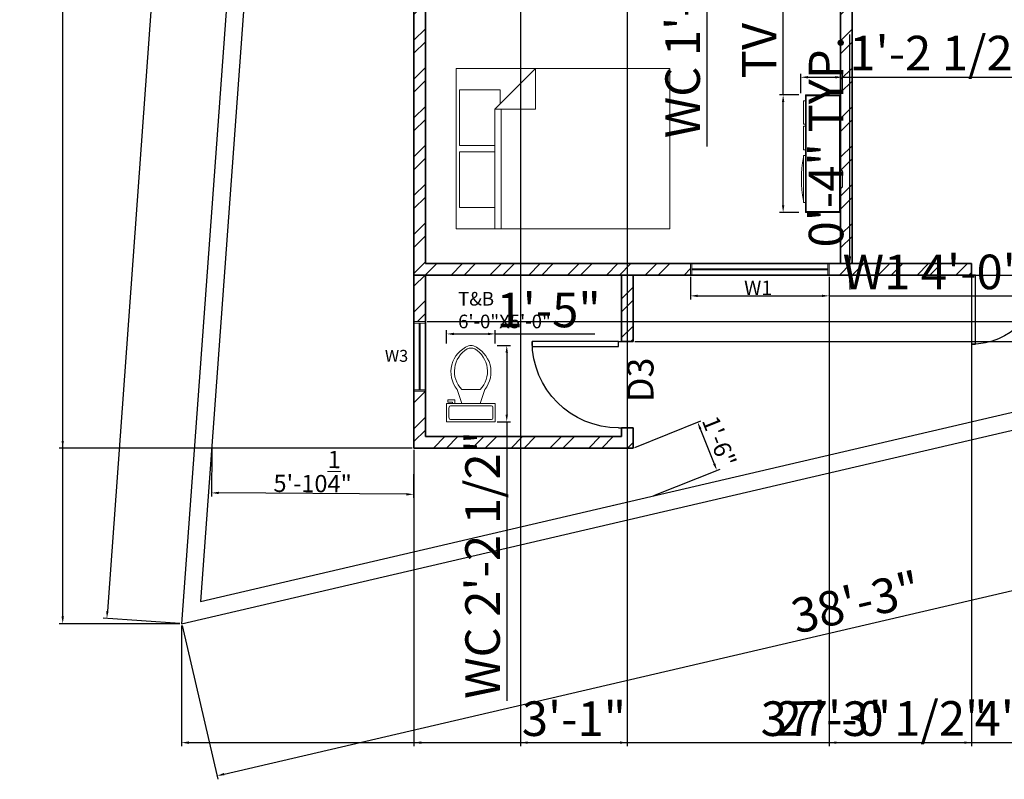
# Model space of a CAD drawing. Units: inches. Extents: x 2242 to 2870, y 1782 to 2635.
# Tile 1 of 7: x 2252 to 2594, y 1782 to 2046. Entities that reach past the tile are written whole.
import ezdxf

# ---------------------------------------------------------------- set-up
doc = ezdxf.new("R2010")
doc.units = ezdxf.units.IN
for name, color, linetype, lineweight in [('A-ANNO-DIMS', 7, 'Continuous', 18), ('A-ANNO-TEXT', 1, 'Continuous', 18), ('A-AREA-IDEN', 1, 'Continuous', 25), ('A-FLOR-FIXT', 9, 'Continuous', 18), ('A-WALL-PATT', 253, 'Continuous', 13), ('C-PROP', 7, 'Continuous', 30), ('doors', 5, 'Continuous', 25), ('furniture', 9, 'Continuous', 18), ('walls', 7, 'Continuous', 35), ('windows', 72, 'Continuous', 18)]:
    doc.layers.add(name, color=color, linetype=linetype, lineweight=lineweight)
doc.styles.get("Standard").update_dxf_attribs({"font": 'arial.ttf'})
doc.dimstyles.new('ISO-25', dxfattribs={"dimtxt": 12, "dimasz": 2.5, "dimexe": 1.25, "dimexo": 0.625, "dimtad": 1, "dimlunit": 4, "dimtxsty": 'Standard', "dimcen": 2.5, "dimadec": 0, "dimazin": 0, "dimtfac": 1, "dimtmove": 0, "dimatfit": 3, "dimfxl": 1, "dimarcsym": 0})

# ---------------------------------------------------------------- blocks, each defined once
blk = doc.blocks.new('*U2')
for p, q in [((0, 0), (0, -5)), ((30, 0), (30, -5))]:
    blk.add_line(p, q)
blk.add_lwpolyline([(0, 0), (0, 30), (1.75, 30), (1.75, 0)], close=True)
blk.add_arc((0, 0), 30, 0, 90)
blk = doc.blocks.new('Bed - Queen')
for p, q in [((0, -80.00003), (0, 0)), ((0, 0), (59.99999, 0)), ((59.99999, 0), (59.99999, -80.00003)), ((7.99999, -1.2), (28.79998, -1.2)), ((7.99999, -14.4), (7.99999, -1.2)), ((28.79998, -1.2), (28.79998, -14.4)), ((31.19999, -1.2), (51.99999, -1.2)), ((31.19999, -14.4), (31.19999, -1.2)), ((51.99999, -1.2), (51.99999, -16.4)), ((0, -14.4), (44.8, -14.4)), ((59.99999, -29.6), (44.8, -14.4)), ((44.8, -14.4), (44.8, -29.6)), ((44.8, -16.8), (0, -16.8)), ((51.99999, -16.4), (46.79936, -16.4)), ((44.8, -29.6), (59.99999, -29.6)), ((59.99999, -80.00003), (0, -80.00003))]:
    blk.add_line(p, q)
blk = doc.blocks.new('Toilet - top')
for p, q in [((9.5, -6), (9.5, -2)), ((-10, -8.5), (-8, -8.5)), ((-10, -9.5), (-10, -8.5)), ((-8, -8.5), (-8, -8)), ((-7, -8), (-7, -9.5)), ((-4, -8), (-6, -14)), ((4, -8), (6, -14)), ((-7, -9.5), (-10, -9.5)), ((4, -14), (-4, -14))]:
    blk.add_line(p, q)
blk.add_lwpolyline([(10.5, -8), (10.5, 0), (-10.5, 0), (-10.5, -8)], close=True)
for points in [[(-9.5, -2), (-9.5, -6)], [(8.5, -1), (-8.5, -1)], [(-8.5, -7), (8.5, -7)]]:
    blk.add_lwpolyline(points)
for centre, radius, start, end in [((-8.62, -1.88), 0.884, 81.8699, 188.1301), ((8.62, -1.88), 0.884, 351.8699, 98.1301), ((-8.62, -6.12), 0.884, 171.8699, 278.1301), ((8.62, -6.12), 0.884, 261.8699, 8.1301), ((3.52, -21.58), 12.17, 141.4691, 247.9714), ((4.2, -21.82), 11.33, 136.3677, 238.9468), ((-3.52, -21.58), 12.17, 292.0284, 38.5307), ((-4.2, -21.82), 11.33, 301.053, 43.6321), ((0, -27.88), 4, 245.7318, 294.2682), ((0, -29), 4, 254.8605, 285.1395)]:
    blk.add_arc(centre, radius, start, end)
blk = doc.blocks.new('Entertainment Center')
for p, q in [((-4, 0), (-5, -1)), ((4, 0), (-4, 0)), ((5, -1), (4, 0)), ((-17, -19), (-17, -1)), ((-17, -1), (43, -1)), ((-16.5, -18.5), (-16.5, -1.5)), ((-16.5, -1.5), (42.5, -1.5)), ((42.5, -1.5), (42.5, -18.5)), ((43, -1), (43, -19)), ((43, -19), (-17, -19)), ((42.5, -18.5), (-16.5, -18.5)), ((-12, -20), (-12, -19)), ((12, -20), (-12, -20)), ((12, -19), (12, -20)), ((15, -20), (15, -19)), ((27, -20), (15, -20)), ((27, -19), (27, -20)), ((28, -20), (28, -19)), ((40, -20), (28, -20)), ((40, -19), (40, -20))]:
    blk.add_line(p, q)
blk.add_arc((0, 40), 61, 259.6111, 280.3889)
blk = doc.blocks.new('*D16')
at = {"layer": 'A-ANNO-DIMS', "color": 0, "lineweight": -2, "transparency": 16777216}
for p, q in [((2358.54, 2540.38), (2331.98, 2542.3)), ((2333.04, 2539.72), (2282.38, 1840.55)), ((2307.51, 1836.23), (2280.95, 1838.15))]:
    blk.add_line(p, q, dxfattribs=at)
at = {"layer": 'A-ANNO-DIMS', "color": 0, "transparency": 16777216}
for points in [[(2332.63, 2539.75), (2333.46, 2539.69), (2333.22, 2542.21)], [(2281.96, 1840.58), (2282.79, 1840.52), (2282.2, 1838.06)]]:
    blk.add_solid(points, dxfattribs=at)
at = {"layer": 'Defpoints', "color": 0, "transparency": 16777216}
for p in [(2359.16, 2540.33), (2282.2, 1838.06), (2308.14, 1836.18)]:
    blk.add_point(p, dxfattribs=at)
at = {"layer": 'A-ANNO-DIMS', "color": 0, "transparency": 16777216, "insert": (2300.98, 2190.63), "char_height": 12, "attachment_point": 5, "rotation": 85.8553}
blk.add_mtext('58\'-10"', dxfattribs=at)
blk = doc.blocks.new('*D17')
at = {"layer": 'A-ANNO-DIMS', "color": 0, "lineweight": -2, "transparency": 16777216}
for p, q in [((2755.31, 1939.73), (2767.74, 1886.37)), ((2322.86, 1784), (2765.02, 1887.02)), ((2308.28, 1835.57), (2320.71, 1782.21))]:
    blk.add_line(p, q, dxfattribs=at)
at = {"layer": 'A-ANNO-DIMS', "color": 0, "transparency": 16777216}
for points in [[(2764.92, 1887.42), (2765.11, 1886.61), (2767.45, 1887.58)], [(2322.77, 1784.4), (2322.96, 1783.59), (2320.43, 1783.43)]]:
    blk.add_solid(points, dxfattribs=at)
at = {"layer": 'Defpoints', "color": 0, "transparency": 16777216}
for p in [(2755.16, 1940.33), (2767.45, 1887.58), (2308.14, 1836.18)]:
    blk.add_point(p, dxfattribs=at)
at = {"layer": 'A-ANNO-DIMS', "color": 0, "transparency": 16777216, "insert": (2542.41, 1842.09), "char_height": 12, "attachment_point": 5, "rotation": 13.1155}
blk.add_mtext('38\'-3"', dxfattribs=at)
blk = doc.blocks.new('*D18')
at = {"layer": 'A-ANNO-DIMS', "color": 0, "lineweight": -2, "transparency": 16777216}
for p, q in [((2465.32, 1897.33), (2488.32, 1906.52)), ((2488.08, 1903.73), (2492.91, 1891.67)), ((2472, 1880.62), (2495, 1889.81))]:
    blk.add_line(p, q, dxfattribs=at)
at = {"layer": 'A-ANNO-DIMS', "color": 0, "transparency": 16777216}
for points in [[(2488.47, 1903.89), (2487.7, 1903.58), (2487.16, 1906.06)], [(2493.29, 1891.82), (2492.52, 1891.51), (2493.84, 1889.34)]]:
    blk.add_solid(points, dxfattribs=at)
at = {"layer": 'Defpoints', "color": 0, "transparency": 16777216}
for p in [(2464.74, 1897.1), (2493.84, 1889.34), (2471.42, 1880.39)]:
    blk.add_point(p, dxfattribs=at)
at = {"layer": 'A-ANNO-DIMS', "color": 0, "transparency": 16777216, "insert": (2493.92, 1899.07), "char_height": 6, "attachment_point": 5, "rotation": 291.788}
blk.add_mtext('1\'-6"', dxfattribs=at)
blk = doc.blocks.new('*D20')
at = {"layer": 'A-ANNO-DIMS', "color": 0, "lineweight": -2, "transparency": 16777216}
for p, q in [((2318.6, 1896.99), (2318.48, 1880.3)), ((2388.74, 1896.47), (2388.62, 1879.78)), ((2386.13, 1881.05), (2320.99, 1881.53))]:
    blk.add_line(p, q, dxfattribs=at)
at = {"layer": 'A-ANNO-DIMS', "color": 0, "transparency": 16777216}
for points in [[(2320.99, 1881.95), (2320.98, 1881.11), (2318.49, 1881.55)], [(2386.13, 1881.47), (2386.12, 1880.63), (2388.63, 1881.03)]]:
    blk.add_solid(points, dxfattribs=at)
at = {"layer": 'Defpoints', "color": 0, "transparency": 16777216}
for p in [(2318.6, 1897.61), (2388.74, 1897.1), (2318.49, 1881.55)]:
    blk.add_point(p, dxfattribs=at)
at = {"layer": 'A-ANNO-DIMS', "color": 0, "transparency": 16777216, "insert": (2353.61, 1888.98), "char_height": 6, "attachment_point": 5, "rotation": 359.5783}
blk.add_mtext('5\'-10{\\H1x;\\S1/4;}"', dxfattribs=at)
blk = doc.blocks.new('WIN-W3-24IN')
for p, q in [((0, 0), (0, 24.12)), ((0, 24.12), (4, 24.12)), ((4, 24.12), (4, 0)), ((0, 23.62), (4, 23.62)), ((1.8, 23.62), (1.8, 0.5)), ((2.2, 23.62), (2.2, 0.5)), ((4, 0.5), (0, 0.5)), ((4, 0), (0, 0))]:
    blk.add_line(p, q)
blk = doc.blocks.new('WIN-W1-48IN')
for p, q in [((0, 4), (48.12, 4)), ((0, 0), (0, 4)), ((0.5, 0), (0.5, 4)), ((47.62, 4), (47.62, 0)), ((48.12, 4), (48.12, 0)), ((48.12, 0), (0, 0)), ((0.5, 2.2), (47.62, 2.2)), ((0.5, 1.8), (47.62, 1.8))]:
    blk.add_line(p, q)
blk = doc.blocks.new('*D35')
at = {"layer": 'A-ANNO-DIMS', "color": 0, "lineweight": -2, "transparency": 16777216}
for p, q in [((2484.67, 1956.47), (2484.67, 1948.63)), ((2532.79, 1956.47), (2532.79, 1948.63)), ((2487.17, 1949.88), (2530.29, 1949.88)), ((2532.79, 1949.88), (2639.98, 1949.88))]:
    blk.add_line(p, q, dxfattribs=at)
at = {"layer": 'A-ANNO-DIMS', "color": 0, "transparency": 16777216}
for points in [[(2487.17, 1950.3), (2487.17, 1949.46), (2484.67, 1949.88)], [(2530.29, 1950.3), (2530.29, 1949.46), (2532.79, 1949.88)]]:
    blk.add_solid(points, dxfattribs=at)
at = {"layer": 'Defpoints', "color": 0, "transparency": 16777216}
for p in [(2484.67, 1957.1), (2532.79, 1957.1), (2532.79, 1949.88)]:
    blk.add_point(p, dxfattribs=at)
at = {"layer": 'A-ANNO-DIMS', "color": 0, "transparency": 16777216, "insert": (2587.64, 1956.63), "char_height": 12, "attachment_point": 5}
blk.add_mtext('W1 4\'-0" TYP.', dxfattribs=at)
blk = doc.blocks.new('*D36')
at = {"layer": 'A-ANNO-DIMS', "color": 0, "lineweight": -2, "transparency": 16777216}
for p, q in [((2540.01, 1963.6), (2540.01, 2040.49)), ((2533.41, 1961.1), (2541.26, 1961.1)), ((2540.01, 1957.1), (2540.01, 1961.1)), ((2533.41, 1957.1), (2541.26, 1957.1)), ((2540.01, 1954.6), (2540.01, 1952.1))]:
    blk.add_line(p, q, dxfattribs=at)
at = {"layer": 'A-ANNO-DIMS', "color": 0, "transparency": 16777216}
for points in [[(2539.59, 1963.6), (2540.42, 1963.6), (2540.01, 1961.1)], [(2539.59, 1954.6), (2540.42, 1954.6), (2540.01, 1957.1)]]:
    blk.add_solid(points, dxfattribs=at)
at = {"layer": 'Defpoints', "color": 0, "transparency": 16777216}
for p in [(2532.79, 1961.1), (2540.01, 1961.1), (2532.79, 1957.1)]:
    blk.add_point(p, dxfattribs=at)
at = {"layer": 'A-ANNO-DIMS', "color": 0, "transparency": 16777216, "insert": (2533.26, 2003.3), "char_height": 12, "attachment_point": 5, "rotation": 90}
blk.add_mtext('0\'-4" TYP.', dxfattribs=at)
blk = doc.blocks.new('*D41')
at = {"layer": 'A-ANNO-DIMS', "color": 0, "lineweight": -2, "transparency": 16777216}
for p, q in [((2516.82, 2019.58), (2516.82, 2166.63)), ((2522.31, 2019.58), (2515.57, 2019.58)), ((2516.82, 1981.32), (2516.82, 2017.08)), ((2522.31, 1978.82), (2515.57, 1978.82))]:
    blk.add_line(p, q, dxfattribs=at)
at = {"layer": 'A-ANNO-DIMS', "color": 0, "transparency": 16777216}
for points in [[(2516.4, 2017.08), (2517.23, 2017.08), (2516.82, 2019.58)], [(2516.4, 1981.32), (2517.23, 1981.32), (2516.82, 1978.82)]]:
    blk.add_solid(points, dxfattribs=at)
at = {"layer": 'Defpoints', "color": 0, "transparency": 16777216}
for p in [(2516.82, 2019.58), (2522.93, 2019.58), (2522.93, 1978.82)]:
    blk.add_point(p, dxfattribs=at)
at = {"layer": 'A-ANNO-DIMS', "color": 0, "transparency": 16777216, "insert": (2510.06, 2094.35), "char_height": 12, "attachment_point": 5, "rotation": 90}
blk.add_mtext('TV UNIT 3\'-5" TYP.', dxfattribs=at)
blk = doc.blocks.new('*D42')
at = {"layer": 'A-ANNO-DIMS', "color": 0, "lineweight": -2, "transparency": 16777216}
for p, q in [((2522.93, 2020.21), (2522.93, 2026.94)), ((2525.43, 2025.69), (2534.92, 2025.69)), ((2537.42, 2020.21), (2537.42, 2026.94)), ((2537.42, 2025.69), (2641.15, 2025.69))]:
    blk.add_line(p, q, dxfattribs=at)
at = {"layer": 'A-ANNO-DIMS', "color": 0, "transparency": 16777216}
for points in [[(2525.43, 2026.11), (2525.43, 2025.28), (2522.93, 2025.69)], [(2534.92, 2026.11), (2534.92, 2025.28), (2537.42, 2025.69)]]:
    blk.add_solid(points, dxfattribs=at)
at = {"layer": 'Defpoints', "color": 0, "transparency": 16777216}
for p in [(2537.42, 2025.69), (2522.93, 2019.58), (2537.42, 2019.58)]:
    blk.add_point(p, dxfattribs=at)
at = {"layer": 'A-ANNO-DIMS', "color": 0, "transparency": 16777216, "insert": (2590.54, 2032.52), "char_height": 12, "attachment_point": 5}
blk.add_mtext('1\'-2 1/2" TYP.', dxfattribs=at)
blk = doc.blocks.new('*D47')
at = {"layer": 'A-ANNO-DIMS', "color": 0, "lineweight": -2, "transparency": 16777216}
for p, q in [((2417.57, 1932.69), (2422.18, 1932.69)), ((2420.93, 1930.19), (2420.93, 1908.65)), ((2417.57, 1906.15), (2422.18, 1906.15)), ((2420.93, 1906.15), (2420.93, 1809.46))]:
    blk.add_line(p, q, dxfattribs=at)
at = {"layer": 'A-ANNO-DIMS', "color": 0, "transparency": 16777216}
for points in [[(2420.51, 1930.19), (2421.35, 1930.19), (2420.93, 1932.69)], [(2420.51, 1908.65), (2421.35, 1908.65), (2420.93, 1906.15)]]:
    blk.add_solid(points, dxfattribs=at)
at = {"layer": 'Defpoints', "color": 0, "transparency": 16777216}
for p in [(2416.95, 1932.69), (2416.95, 1906.15), (2420.93, 1906.15)]:
    blk.add_point(p, dxfattribs=at)
at = {"layer": 'A-ANNO-DIMS', "color": 0, "transparency": 16777216, "insert": (2414.1, 1856.56), "char_height": 12, "attachment_point": 5, "rotation": 90}
blk.add_mtext('WC 2\'-2 1/2"', dxfattribs=at)
blk = doc.blocks.new('*D48')
at = {"layer": 'A-ANNO-DIMS', "color": 0, "lineweight": -2, "transparency": 16777216}
for p, q in [((2400.08, 1933.32), (2400.08, 1937.93)), ((2416.95, 1933.32), (2416.95, 1937.93)), ((2402.58, 1936.68), (2414.45, 1936.68)), ((2416.95, 1936.68), (2451.47, 1936.68))]:
    blk.add_line(p, q, dxfattribs=at)
at = {"layer": 'A-ANNO-DIMS', "color": 0, "transparency": 16777216}
for points in [[(2402.58, 1937.09), (2402.58, 1936.26), (2400.08, 1936.68)], [(2414.45, 1937.09), (2414.45, 1936.26), (2416.95, 1936.68)]]:
    blk.add_solid(points, dxfattribs=at)
at = {"layer": 'Defpoints', "color": 0, "transparency": 16777216}
for p in [(2416.95, 1936.68), (2400.08, 1932.69), (2416.95, 1932.69)]:
    blk.add_point(p, dxfattribs=at)
at = {"layer": 'A-ANNO-DIMS', "color": 0, "transparency": 16777216, "insert": (2435.46, 1943.43), "char_height": 12, "attachment_point": 5}
blk.add_mtext('1\'-5"', dxfattribs=at)
blk = doc.blocks.new('*D49')
at = {"layer": 'A-ANNO-DIMS', "color": 0, "lineweight": -2, "transparency": 16777216}
for p, q in [((2487.98, 2131.46), (2491.58, 2131.46)), ((2490.33, 2128.96), (2490.33, 2114.14)), ((2487.98, 2111.64), (2491.58, 2111.64)), ((2490.33, 2111.64), (2490.33, 2001.67))]:
    blk.add_line(p, q, dxfattribs=at)
at = {"layer": 'A-ANNO-DIMS', "color": 0, "transparency": 16777216}
for points in [[(2489.91, 2128.96), (2490.75, 2128.96), (2490.33, 2131.46)], [(2489.91, 2114.14), (2490.75, 2114.14), (2490.33, 2111.64)]]:
    blk.add_solid(points, dxfattribs=at)
at = {"layer": 'Defpoints', "color": 0, "transparency": 16777216}
for p in [(2487.36, 2131.46), (2487.36, 2111.64), (2490.33, 2111.64)]:
    blk.add_point(p, dxfattribs=at)
at = {"layer": 'A-ANNO-DIMS', "color": 0, "transparency": 16777216, "insert": (2483.5, 2055.41), "char_height": 12, "attachment_point": 5, "rotation": 90}
blk.add_mtext('WC 1\'-8" TYP.', dxfattribs=at)
blk = doc.blocks.new('*D55')
at = {"layer": 'A-ANNO-DIMS', "color": 0, "lineweight": -2, "transparency": 16777216}
for p, q in [((2358.54, 2540.33), (2265.64, 2540.33)), ((2266.89, 1838.68), (2266.89, 2537.83)), ((2307.51, 1836.18), (2265.64, 1836.18))]:
    blk.add_line(p, q, dxfattribs=at)
at = {"layer": 'A-ANNO-DIMS', "color": 0, "transparency": 16777216}
for points in [[(2266.47, 2537.83), (2267.3, 2537.83), (2266.89, 2540.33)], [(2266.47, 1838.68), (2267.3, 1838.68), (2266.89, 1836.18)]]:
    blk.add_solid(points, dxfattribs=at)
at = {"layer": 'Defpoints', "color": 0, "transparency": 16777216}
for p in [(2266.89, 2540.33), (2359.16, 2540.33), (2308.14, 1836.18)]:
    blk.add_point(p, dxfattribs=at)
at = {"layer": 'A-ANNO-DIMS', "color": 0, "transparency": 16777216, "insert": (2260.13, 2188.26), "char_height": 12, "attachment_point": 5, "rotation": 90}
blk.add_mtext('58\'-8"', dxfattribs=at)
blk = doc.blocks.new('*D56')
at = {"layer": 'A-ANNO-DIMS', "color": 0, "lineweight": -2, "transparency": 16777216}
for p, q in [((2755.16, 1939.71), (2755.16, 1793.68)), ((2308.14, 1835.56), (2308.14, 1793.68)), ((2310.64, 1794.93), (2752.66, 1794.93))]:
    blk.add_line(p, q, dxfattribs=at)
at = {"layer": 'A-ANNO-DIMS', "color": 0, "transparency": 16777216}
for points in [[(2310.64, 1795.35), (2310.64, 1794.51), (2308.14, 1794.93)], [(2752.66, 1795.35), (2752.66, 1794.51), (2755.16, 1794.93)]]:
    blk.add_solid(points, dxfattribs=at)
at = {"layer": 'Defpoints', "color": 0, "transparency": 16777216}
for p in [(2755.16, 1940.33), (2308.14, 1836.18), (2755.16, 1794.93)]:
    blk.add_point(p, dxfattribs=at)
at = {"layer": 'A-ANNO-DIMS', "color": 0, "transparency": 16777216, "insert": (2531.65, 1801.69), "char_height": 12, "attachment_point": 5}
blk.add_mtext('37\'-3"', dxfattribs=at)
blk = doc.blocks.new('*D57')
at = {"layer": 'A-ANNO-DIMS', "color": 0, "lineweight": -2, "transparency": 16777216}
for p, q in [((2713.16, 1956.47), (2713.16, 1793.68)), ((2388.74, 1896.47), (2388.74, 1793.68)), ((2391.24, 1794.93), (2710.66, 1794.93))]:
    blk.add_line(p, q, dxfattribs=at)
at = {"layer": 'A-ANNO-DIMS', "color": 0, "transparency": 16777216}
for points in [[(2391.24, 1795.35), (2391.24, 1794.51), (2388.74, 1794.93)], [(2710.66, 1795.35), (2710.66, 1794.51), (2713.16, 1794.93)]]:
    blk.add_solid(points, dxfattribs=at)
at = {"layer": 'Defpoints', "color": 0, "transparency": 16777216}
for p in [(2713.16, 1957.1), (2388.74, 1897.1), (2713.16, 1794.93)]:
    blk.add_point(p, dxfattribs=at)
at = {"layer": 'A-ANNO-DIMS', "color": 0, "transparency": 16777216, "insert": (2550.95, 1801.76), "char_height": 12, "attachment_point": 5}
blk.add_mtext('27\'-0 1/2"', dxfattribs=at)
blk = doc.blocks.new('*D58')
at = {"layer": 'A-ANNO-DIMS', "color": 0, "lineweight": -2, "transparency": 16777216}
for p, q in [((2388.12, 2433.1), (2265.64, 2433.1)), ((2266.89, 1899.6), (2266.89, 2430.6)), ((2388.12, 1897.1), (2265.64, 1897.1))]:
    blk.add_line(p, q, dxfattribs=at)
at = {"layer": 'A-ANNO-DIMS', "color": 0, "transparency": 16777216}
for points in [[(2266.47, 2430.6), (2267.3, 2430.6), (2266.89, 2433.1)], [(2266.47, 1899.6), (2267.3, 1899.6), (2266.89, 1897.1)]]:
    blk.add_solid(points, dxfattribs=at)
at = {"layer": 'Defpoints', "color": 0, "transparency": 16777216}
for p in [(2266.89, 2433.1), (2388.74, 2433.1), (2388.74, 1897.1)]:
    blk.add_point(p, dxfattribs=at)
at = {"layer": 'A-ANNO-DIMS', "color": 0, "transparency": 16777216, "insert": (2260.13, 2165.1), "char_height": 12, "attachment_point": 5, "rotation": 90}
blk.add_mtext('44\'-8"', dxfattribs=at)
blk = doc.blocks.new('*D72')
at = {"layer": 'A-ANNO-DIMS', "color": 0, "lineweight": -2, "transparency": 16777216}
for p, q in [((2532.79, 1956.47), (2532.79, 1793.68)), ((2582.16, 1956.47), (2582.16, 1793.68)), ((2535.29, 1794.93), (2579.66, 1794.93)), ((2582.16, 1794.93), (2646.26, 1794.93))]:
    blk.add_line(p, q, dxfattribs=at)
at = {"layer": 'A-ANNO-DIMS', "color": 0, "transparency": 16777216}
for points in [[(2535.29, 1795.35), (2535.29, 1794.51), (2532.79, 1794.93)], [(2579.66, 1795.35), (2579.66, 1794.51), (2582.16, 1794.93)]]:
    blk.add_solid(points, dxfattribs=at)
at = {"layer": 'Defpoints', "color": 0, "transparency": 16777216}
for p in [(2532.79, 1957.1), (2582.16, 1957.1), (2582.16, 1794.93)]:
    blk.add_point(p, dxfattribs=at)
at = {"layer": 'A-ANNO-DIMS', "color": 0, "transparency": 16777216, "insert": (2615.46, 1801.76), "char_height": 12, "attachment_point": 5}
blk.add_mtext('4\'-1 1/2"', dxfattribs=at)
blk = doc.blocks.new('*D76')
at = {"layer": 'A-ANNO-DIMS', "color": 0, "lineweight": -2, "transparency": 16777216}
for p, q in [((2796.41, 1957.1), (2796.41, 1991.62)), ((2393.37, 1957.1), (2797.66, 1957.1)), ((2796.41, 1943.45), (2796.41, 1954.6)), ((2393.37, 1940.95), (2797.66, 1940.95))]:
    blk.add_line(p, q, dxfattribs=at)
at = {"layer": 'A-ANNO-DIMS', "color": 0, "transparency": 16777216}
for points in [[(2796, 1954.6), (2796.83, 1954.6), (2796.41, 1957.1)], [(2796, 1943.45), (2796.83, 1943.45), (2796.41, 1940.95)]]:
    blk.add_solid(points, dxfattribs=at)
at = {"layer": 'Defpoints', "color": 0, "transparency": 16777216}
for p in [(2392.74, 1957.1), (2796.41, 1957.1), (2392.74, 1940.95)]:
    blk.add_point(p, dxfattribs=at)
at = {"layer": 'A-ANNO-DIMS', "color": 0, "transparency": 16777216, "insert": (2789.76, 1975.61), "char_height": 12, "attachment_point": 5, "rotation": 90}
blk.add_mtext('1\'-4"', dxfattribs=at)
blk = doc.blocks.new('*D85')
at = {"layer": 'A-ANNO-DIMS', "color": 0, "lineweight": -2, "transparency": 16777216}
for p, q in [((2465.37, 1957.1), (2797.66, 1957.1)), ((2796.41, 1954.6), (2796.41, 1936.6)), ((2465.37, 1934.1), (2797.66, 1934.1)), ((2796.41, 1934.1), (2796.41, 1890.25))]:
    blk.add_line(p, q, dxfattribs=at)
at = {"layer": 'A-ANNO-DIMS', "color": 0, "transparency": 16777216}
for points in [[(2796, 1954.6), (2796.83, 1954.6), (2796.41, 1957.1)], [(2796, 1936.6), (2796.83, 1936.6), (2796.41, 1934.1)]]:
    blk.add_solid(points, dxfattribs=at)
at = {"layer": 'Defpoints', "color": 0, "transparency": 16777216}
for p in [(2464.74, 1957.1), (2464.74, 1934.1), (2796.41, 1934.1)]:
    blk.add_point(p, dxfattribs=at)
at = {"layer": 'A-ANNO-DIMS', "color": 0, "transparency": 16777216, "insert": (2789.76, 1910.93), "char_height": 12, "attachment_point": 5, "rotation": 90}
blk.add_mtext('1\'-11"', dxfattribs=at)
blk = doc.blocks.new('*D86')
at = {"layer": 'A-ANNO-DIMS', "color": 0, "lineweight": -2, "transparency": 16777216}
for p, q in [((2425.74, 2108.47), (2425.74, 1793.68)), ((2462.74, 2108.47), (2462.74, 1793.68)), ((2428.24, 1794.93), (2460.24, 1794.93))]:
    blk.add_line(p, q, dxfattribs=at)
at = {"layer": 'A-ANNO-DIMS', "color": 0, "transparency": 16777216}
for points in [[(2428.24, 1795.35), (2428.24, 1794.51), (2425.74, 1794.93)], [(2460.24, 1795.35), (2460.24, 1794.51), (2462.74, 1794.93)]]:
    blk.add_solid(points, dxfattribs=at)
at = {"layer": 'Defpoints', "color": 0, "transparency": 16777216}
for p in [(2425.74, 2109.1), (2462.74, 2109.1), (2462.74, 1794.93)]:
    blk.add_point(p, dxfattribs=at)
at = {"layer": 'A-ANNO-DIMS', "color": 0, "transparency": 16777216, "insert": (2444.24, 1801.69), "char_height": 12, "attachment_point": 5}
blk.add_mtext('3\'-1"', dxfattribs=at)

msp = doc.modelspace()

# ---------------------------------------------------------------- hatches: boundary and pattern name
at = {"layer": 'A-WALL-PATT'}
h = msp.add_hatch(dxfattribs=at)
h.set_pattern_fill('ANSI32', color=256)
h.paths.add_polyline_path([(2392.745, 2066.174), (2388.745, 2066.174), (2388.745, 1957.097), (2484.674, 1957.097), (2484.674, 1961.097), (2392.745, 1961.097)])
h = msp.add_hatch(dxfattribs=at)
h.set_pattern_fill('ANSI32', color=256)
h.paths.add_polyline_path([(2540.745, 2066.097), (2536.745, 2066.097), (2536.745, 1993.766), (2537.424, 1993.086), (2537.424, 1987.651), (2536.745, 1986.972), (2536.745, 1978.82), (2536.745, 1961.097), (2540.745, 1961.097)])
h = msp.add_hatch(dxfattribs=at)
h.set_pattern_fill('ANSI32', color=256)
h.paths.add_polyline_path([(2582.164, 1961.097), (2532.79, 1961.097), (2532.79, 1957.097), (2582.164, 1957.097)])
h = msp.add_hatch(dxfattribs=at)
h.set_pattern_fill('ANSI32', color=256)
h.paths.add_polyline_path([(2392.745, 1957.097), (2388.745, 1957.097), (2388.745, 1940.946), (2392.745, 1940.946)])
h = msp.add_hatch(dxfattribs=at)
h.set_pattern_fill('ANSI32', color=256)
h.paths.add_polyline_path([(2464.745, 1957.097), (2460.745, 1957.097), (2460.745, 1934.097), (2464.745, 1934.097)])
h = msp.add_hatch(dxfattribs=at)
h.set_pattern_fill('ANSI32', color=256)
h.paths.add_polyline_path([(2464.745, 1904.097), (2460.745, 1904.097), (2460.745, 1901.097), (2392.745, 1901.097), (2392.745, 1916.83), (2388.745, 1916.83), (2388.745, 1897.097), (2464.745, 1897.097)])

# ---------------------------------------------------------------- linework, layer by layer
at = {"layer": 'C-PROP'}
for p, q in [((2359.164, 2540.335), (2308.137, 1836.181)), ((2364.745, 2534.335), (2314.71, 1843.873)), ((2314.71, 1843.873), (2749.164, 1945.097)), ((2308.137, 1836.181), (2755.164, 1940.335))]:
    msp.add_line(p, q, dxfattribs=at)
at = {"layer": 'walls'}
for p, q in [((2388.745, 1957.097), (2388.745, 2433.097)), ((2392.745, 1961.097), (2392.745, 2429.097)), ((2536.745, 1961.097), (2536.745, 2066.097)), ((2540.745, 1961.097), (2540.745, 2066.097)), ((2582.164, 1961.097), (2392.745, 1961.097)), ((2582.164, 1957.097), (2582.164, 1961.097)), ((2388.745, 1957.097), (2388.745, 1897.097)), ((2582.164, 1957.097), (2388.745, 1957.097)), ((2392.745, 1957.097), (2392.745, 1901.097)), ((2460.745, 1934.097), (2460.745, 1957.097)), ((2464.745, 1934.097), (2464.745, 1957.097)), ((2464.745, 1934.097), (2460.745, 1934.097)), ((2460.745, 1901.097), (2460.745, 1904.097)), ((2460.745, 1901.097), (2460.745, 1904.097)), ((2460.745, 1904.097), (2464.745, 1904.097)), ((2464.745, 1897.097), (2464.745, 1904.097)), ((2392.745, 1901.097), (2460.745, 1901.097)), ((2388.745, 1897.097), (2464.745, 1897.097))]:
    msp.add_line(p, q, dxfattribs=at)

# ---------------------------------------------------------------- block references
at = {"layer": 'A-FLOR-FIXT', "xscale": -0.8031669041615042, "yscale": 0.8031669041615042, "zscale": 0.8031669041615042, "rotation": 180}
msp.add_blockref('Toilet - top', (2408.514, 1906.152), dxfattribs=at)
at = {"layer": 'doors', "xscale": -0.8, "yscale": 0.8, "zscale": 0.8, "rotation": 180}
msp.add_blockref('*U2', (2582.164, 1957.097), dxfattribs=at)
at = {"layer": 'doors', "xscale": -1, "rotation": 90}
msp.add_blockref('*U2', (2459.745, 1934.097), dxfattribs=at)
at = {"layer": 'furniture'}
for name, p, xscale, yscale, zscale, rotation in [('Bed - Queen', (2403.439, 1973.16), 0.9262549739508827, 0.9262549739508827, 0.9262549739508827, 90), ('Entertainment Center', (2537.424, 1990.369), -0.6793374069686555, 0.6793374069686555, 0.6793374069686555, 270)]:
    msp.add_blockref(name, p, dxfattribs=dict(at, xscale=xscale, yscale=yscale, zscale=zscale, rotation=rotation))
at = {"layer": 'windows'}
msp.add_blockref('WIN-W1-48IN', (2484.674, 1957.097), dxfattribs=at)
at = {"layer": 'windows', "rotation": 180}
msp.add_blockref('WIN-W3-24IN', (2392.744, 1940.946), dxfattribs=at)

# ---------------------------------------------------------------- texts
at = {"layer": 'A-ANNO-TEXT', "attachment_point": 1}
for s, width, gutter_width, insert, char_height in [('W1', 1.76313, 25, (2503.263, 1955.179), 5), ('W3', 1.14454, 20.658, (2378.657, 1931.132), 4.1316)]:
    msp.add_mtext_dynamic_manual_height_columns(s, width=width, gutter_width=gutter_width, heights=[0], dxfattribs=dict(at, insert=insert, char_height=char_height))
at = {"layer": 'A-ANNO-TEXT', "insert": (2462.732, 1913.02), "char_height": 9.1137, "attachment_point": 1, "rotation": 90}
msp.add_mtext_dynamic_manual_height_columns('D3', width=1.64651, gutter_width=9.493, heights=[0], dxfattribs=at)
at = {"layer": 'A-AREA-IDEN', "insert": (2404.062, 1951.23), "char_height": 4.72198, "attachment_point": 1}
msp.add_mtext_dynamic_manual_height_columns('T&B\\P6\'-0"X5\'-0"', width=0.50549, gutter_width=23.61, heights=[0], dxfattribs=at)

# ---------------------------------------------------------------- dimensions: what is measured, and where the dimension line sits
at = {"layer": 'A-ANNO-DIMS'}
for p1, p2, distance, override, picture, middle in [((2359.164, 2540.335), (2308.137, 1836.181), -26.007, {"dimclrd": 0, "dimclre": 0, "dimclrt": 0}, '*D16', (2300.976, 2190.626)), ((2308.137, 1836.181), (2755.164, 1940.335), -54.163, {"dimclrd": 0, "dimclre": 0, "dimclrt": 0}, '*D17', (2542.407, 1842.087)), ((2464.745, 1897.097), (2471.424, 1880.386), 24.135, {"dimtxt": 6, "dimclrd": 0, "dimclre": 0, "dimclrt": 0}, '*D18', (2493.92, 1899.069)), ((2388.745, 1897.097), (2318.604, 1897.614), 16.065, {"dimtxt": 6, "dimclrd": 0, "dimclre": 0, "dimclrt": 0}, '*D20', (2353.613, 1888.979))]:
    dim = msp.add_aligned_dim(p1=p1, p2=p2, distance=distance, dimstyle='ISO-25', override=override, dxfattribs=at)
    dim.commit()
    dim.dimension.update_dxf_attribs({"geometry": picture, "text_midpoint": middle})
for base, p1, p2, picture, middle in [((2266.887, 2540.335), (2308.137, 1836.181), (2359.164, 2540.335), '*D55', (2260.135, 2188.258)), ((2266.887, 2433.097), (2388.745, 1897.097), (2388.745, 2433.097), '*D58', (2260.135, 2165.097)), ((2796.414, 1957.097), (2392.745, 1940.946), (2392.745, 1957.097), '*D76', (2789.764, 1975.607)), ((2796.414, 1934.097), (2464.745, 1957.097), (2464.745, 1934.097), '*D85', (2789.764, 1910.926))]:
    dim = msp.add_linear_dim(base=base, p1=p1, p2=p2, angle=90, dimstyle='ISO-25', override={"dimdec": 1, "dimlfac": 1, "dimrnd": 0, "dimzin": 1, "dimdsep": 46, "dimlunit": 4, "dimfrac": 2}, dxfattribs=at)
    dim.commit()
    dim.dimension.update_dxf_attribs({"geometry": picture, "text_midpoint": middle})
for base, p1, p2, angle, text, picture, middle in [((2516.817, 2019.58), (2522.931, 1978.82), (2522.931, 2019.58), 90, 'TV UNIT <> TYP.', '*D41', (2510.061, 2094.353)), ((2490.328, 2111.645), (2487.356, 2131.461), (2487.356, 2111.645), 270, 'WC <> TYP.', '*D49', (2483.499, 2055.408)), ((2540.007, 1961.097), (2532.79, 1957.097), (2532.79, 1961.097), 90, '<> TYP.', '*D36', (2533.256, 2003.295)), ((2420.929, 1906.152), (2416.948, 1932.694), (2416.948, 1906.152), 270, 'WC <>', '*D47', (2414.099, 1856.558))]:
    dim = msp.add_linear_dim(base=base, p1=p1, p2=p2, angle=angle, text=text, dimstyle='ISO-25', override={"dimdec": 1, "dimlfac": 1, "dimrnd": 0, "dimzin": 1, "dimdsep": 46, "dimlunit": 4, "dimfrac": 2}, dxfattribs=at)
    dim.commit()
    dim.dimension.update_dxf_attribs({"geometry": picture, "text_midpoint": middle})
for base, p1, p2, picture, middle in [((2462.745, 1794.931), (2425.745, 2109.097), (2462.745, 2109.097), '*D86', (2444.245, 1801.687)), ((2713.164, 1794.931), (2388.745, 1897.097), (2713.164, 1957.097), '*D57', (2550.954, 1801.761)), ((2582.164, 1794.931), (2532.79, 1957.097), (2582.164, 1957.097), '*D72', (2615.46, 1801.761)), ((2416.948, 1936.675), (2400.081, 1932.694), (2416.948, 1932.694), '*D48', (2435.457, 1943.427)), ((2755.164, 1794.931), (2308.137, 1836.181), (2755.164, 1940.335), '*D56', (2531.65, 1801.687))]:
    dim = msp.add_linear_dim(base=base, p1=p1, p2=p2, dimstyle='ISO-25', override={"dimdec": 1, "dimlfac": 1, "dimrnd": 0, "dimzin": 1, "dimdsep": 46, "dimlunit": 4, "dimfrac": 2}, dxfattribs=at)
    dim.commit()
    dim.dimension.update_dxf_attribs({"geometry": picture, "text_midpoint": middle})
for base, p1, p2, text, picture, middle in [((2537.424, 2025.694), (2522.931, 2019.58), (2537.424, 2019.58), '<> TYP.', '*D42', (2590.538, 2032.524)), ((2532.79, 1949.88), (2484.674, 1957.097), (2532.79, 1957.097), 'W1 <> TYP.', '*D35', (2587.635, 1956.632))]:
    dim = msp.add_linear_dim(base=base, p1=p1, p2=p2, text=text, dimstyle='ISO-25', override={"dimdec": 1, "dimlfac": 1, "dimrnd": 0, "dimzin": 1, "dimdsep": 46, "dimlunit": 4, "dimfrac": 2}, dxfattribs=at)
    dim.commit()
    dim.dimension.update_dxf_attribs({"geometry": picture, "text_midpoint": middle})

doc.saveas('drawing.dxf')
